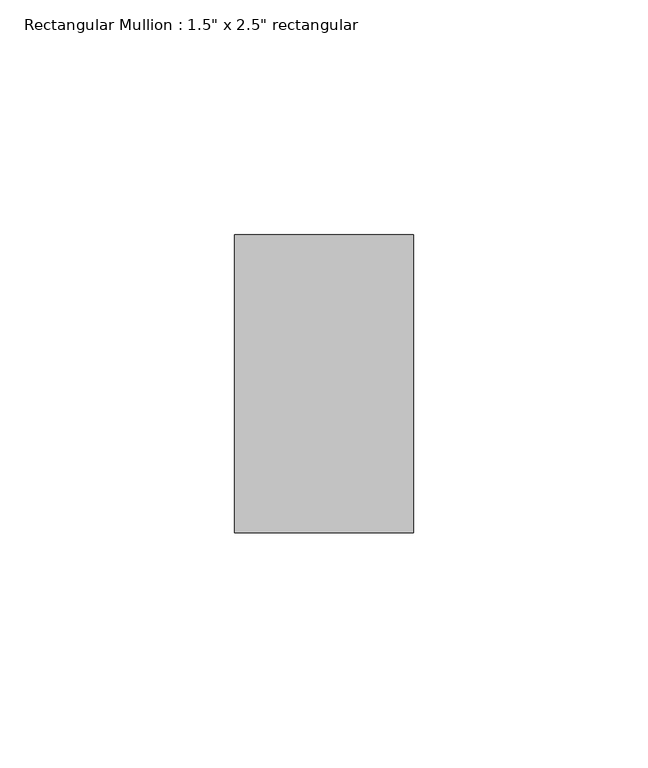
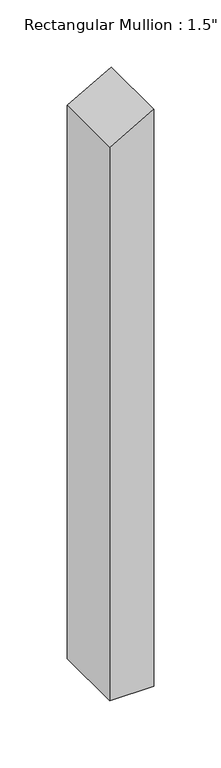
"""IFC4 building model written with IfcOpenShell, lengths in millimetres: member geometry."""

from ifc_helpers import new_model, si_unit, frame, origin, place, context, project, spatial, polyline, outline, extrude, source, transform, mapped, element, save


def member_864d0aaa(model_context):
    return source(origin(), model_context, "Body", "SweptSolid", [
        extrude(outline(polyline([(0.0, 0.0), (-21.676858, -38.1), (-525.3760689, -38.1), (-525.3760689, 0.0), (0.0, 0.0)])), frame((0.0, -31.75, 0.0), z_axis=(0.0, 1.0, 0.0), x_axis=(0.0, 0.0, 1.0)), (0.0, 0.0, 1.0), 63.5),
    ])


if __name__ == "__main__":
    model = new_model("IFC4")
    model_context = context("Model", 3, world=origin())
    ifc_project = project(units=[si_unit("LENGTHUNIT", "METRE", prefix="MILLI")], contexts=[model_context])
    site = spatial("IfcSite", under=ifc_project)
    building = spatial("IfcBuilding", under=site)
    placement = place(None, origin())
    member_shape = member_864d0aaa(model_context)
    element("IfcMember", 1, ObjectType="Rectangular Mullion : 1.5\" x 2.5\" rectangular", at=placement, inside=building, context=model_context, shape_type="MappedRepresentation", body=[
        mapped(member_shape, transform((0.0, 0.0, 0.0), x_axis=(1.0, 0.0, 0.0), y_axis=(0.0, 1.0, 0.0), z_axis=(0.0, 0.0, 1.0))),
    ])
    save(model, "model.ifc")

# Revit data of these elements
# Type "Rectangular Mullion : 1.5\" x 2.5\" rectangular"
#   built-in parameter 1007304 = 0.208333 (stored number, unit not read)
#   built-in parameter 1007301 = 0.0625 (stored number, unit not read)
#   built-in parameter 1007300 = 0.0625 (stored number, unit not read)
